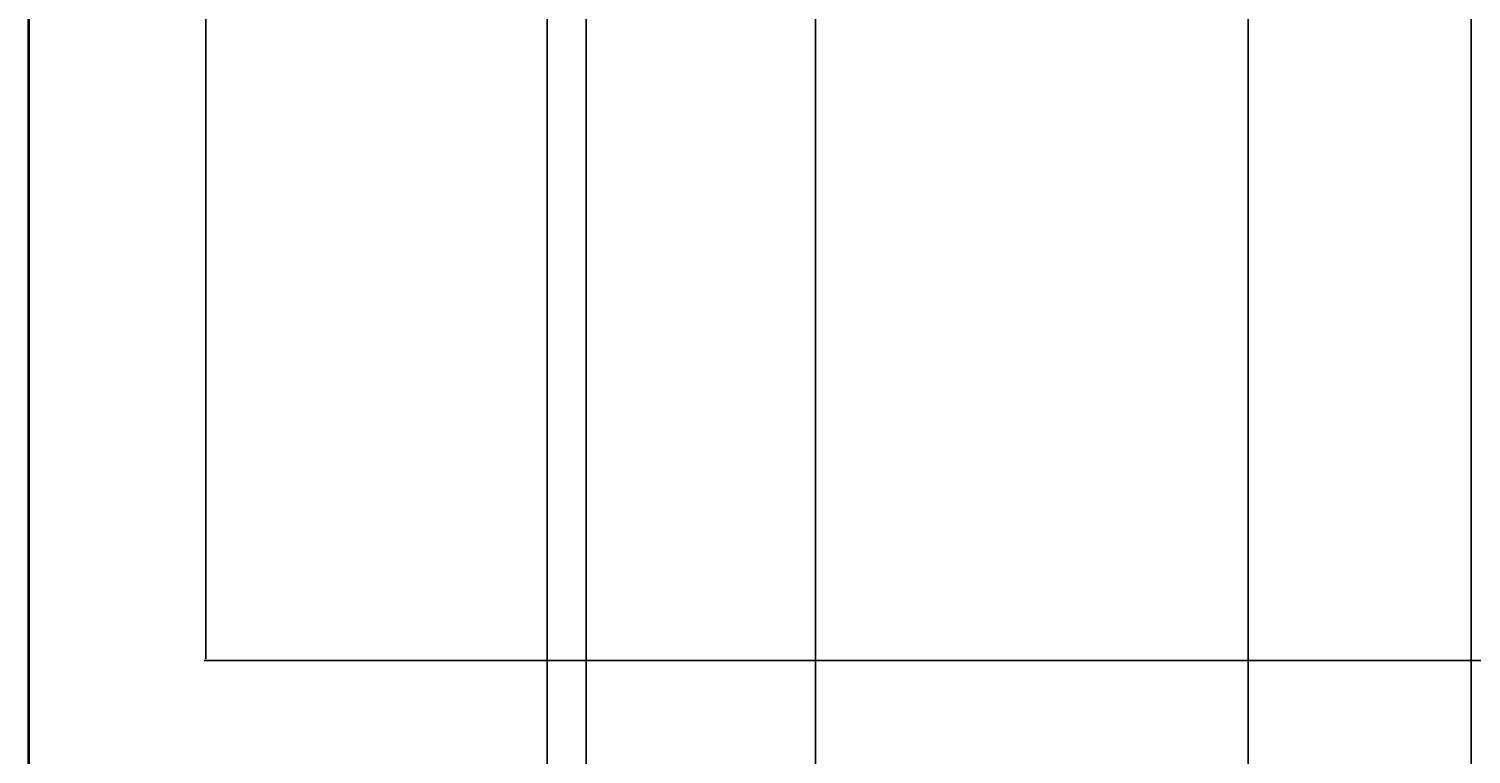
# Model space of a CAD drawing. Units: inches. Extents: x 1734 to 2405, y 1500 to 2491.
# Tile 2 of 14: x 1734 to 1900, y 1700 to 1784. Entities that reach past the tile are written whole.
import ezdxf

# ---------------------------------------------------------------- set-up
doc = ezdxf.new("R2010")
doc.units = ezdxf.units.IN
for name, color, linetype, lineweight in [('A-ANNO-DIMS', 2, 'Continuous', 18), ('A-ANNO-TTLB', 7, 'Continuous', 35), ('C-PROP', 7, 'Continuous', 25)]:
    doc.layers.add(name, color=color, linetype=linetype, lineweight=lineweight)
doc.styles.get("Standard").update_dxf_attribs({"font": 'arial.ttf'})
doc.dimstyles.get("Standard").update_dxf_attribs({"dimtxt": 0.18, "dimasz": 0.18, "dimexe": 0.18, "dimexo": 0.0625, "dimgap": 0.09, "dimtad": 0, "dimtih": 1, "dimtoh": 1, "dimdec": 4, "dimzin": 0, "dimdsep": 46, "dimtxsty": 'Standard', "dimcen": 0.09, "dimadec": 0, "dimazin": 0, "dimtfac": 1, "dimtdec": 4, "dimtofl": 0, "dimtmove": 0, "dimatfit": 3, "dimfxl": 1, "dimtolj": 1, "dimtzin": 0, "dimarcsym": 0})

# ---------------------------------------------------------------- blocks, each defined once
blk = doc.blocks.new('*D23')
at = {"layer": 'A-ANNO-DIMS', "color": 0, "lineweight": -2, "transparency": 16777216}
for p, q in [((1793.83, 2425.82), (1754.36, 2425.82)), ((1754.54, 2425.64), (1754.54, 2068.48)), ((1754.54, 1710.95), (1754.54, 2068.11)), ((1793.83, 1710.77), (1754.36, 1710.77))]:
    blk.add_line(p, q, dxfattribs=at)
at = {"layer": 'A-ANNO-DIMS', "color": 0, "transparency": 16777216}
for points in [[(1754.51, 2425.64), (1754.57, 2425.64), (1754.54, 2425.82)], [(1754.51, 1710.95), (1754.57, 1710.95), (1754.54, 1710.77)]]:
    blk.add_solid(points, dxfattribs=at)
at = {"layer": 'Defpoints', "color": 0, "transparency": 16777216}
for p in [(1754.54, 2425.82), (1793.89, 2425.82), (1793.89, 1710.77)]:
    blk.add_point(p, dxfattribs=at)
at = {"layer": 'A-ANNO-DIMS', "color": 0, "transparency": 16777216, "insert": (1754.54, 2068.3), "char_height": 0.18, "attachment_point": 5}
blk.add_mtext('\\A1;715', dxfattribs=at)
blk = doc.blocks.new('*D24')
at = {"layer": 'A-ANNO-DIMS', "color": 0, "lineweight": -2, "transparency": 16777216}
for p, q in [((1793.89, 1710.7), (1793.89, 1615.47)), ((1900.39, 1710.7), (1900.39, 1615.47)), ((1794.07, 1615.65), (1846.76, 1615.65)), ((1900.21, 1615.65), (1847.53, 1615.65))]:
    blk.add_line(p, q, dxfattribs=at)
at = {"layer": 'A-ANNO-DIMS', "color": 0, "transparency": 16777216}
for points in [[(1794.07, 1615.68), (1794.07, 1615.62), (1793.89, 1615.65)], [(1900.21, 1615.68), (1900.21, 1615.62), (1900.39, 1615.65)]]:
    blk.add_solid(points, dxfattribs=at)
at = {"layer": 'Defpoints', "color": 0, "transparency": 16777216}
for p in [(1793.89, 1710.77), (1900.39, 1710.77), (1900.39, 1615.65)]:
    blk.add_point(p, dxfattribs=at)
at = {"layer": 'A-ANNO-DIMS', "color": 0, "transparency": 16777216, "insert": (1847.14, 1615.65), "char_height": 0.18, "attachment_point": 5}
blk.add_mtext('\\A1;106.5', dxfattribs=at)
blk = doc.blocks.new('*D26')
at = {"layer": 'A-ANNO-DIMS', "color": 0, "lineweight": -2, "transparency": 16777216}
for p, q in [((1900.39, 1798.76), (1900.39, 1615.47)), ((1932.99, 1798.76), (1932.99, 1615.47)), ((1900.57, 1615.65), (1916.37, 1615.65)), ((1932.81, 1615.65), (1917.02, 1615.65))]:
    blk.add_line(p, q, dxfattribs=at)
at = {"layer": 'A-ANNO-DIMS', "color": 0, "transparency": 16777216}
for points in [[(1900.57, 1615.68), (1900.57, 1615.62), (1900.39, 1615.65)], [(1932.81, 1615.68), (1932.81, 1615.62), (1932.99, 1615.65)]]:
    blk.add_solid(points, dxfattribs=at)
at = {"layer": 'Defpoints', "color": 0, "transparency": 16777216}
for p in [(1900.39, 1798.82), (1932.99, 1798.82), (1932.99, 1615.65)]:
    blk.add_point(p, dxfattribs=at)
at = {"layer": 'A-ANNO-DIMS', "color": 0, "transparency": 16777216, "insert": (1916.69, 1615.65), "char_height": 0.18, "attachment_point": 5}
blk.add_mtext('\\A1;32.6', dxfattribs=at)
blk = doc.blocks.new('*D32')
at = {"layer": 'A-ANNO-DIMS', "color": 0, "lineweight": -2, "transparency": 16777216}
for p, q in [((1798.39, 2202.26), (1798.39, 1615.47)), ((1824.83, 2202.26), (1824.83, 1615.47)), ((1798.57, 1615.65), (1811.22, 1615.65)), ((1824.65, 1615.65), (1812.01, 1615.65))]:
    blk.add_line(p, q, dxfattribs=at)
at = {"layer": 'A-ANNO-DIMS', "color": 0, "transparency": 16777216}
for points in [[(1798.57, 1615.68), (1798.57, 1615.62), (1798.39, 1615.65)], [(1824.65, 1615.68), (1824.65, 1615.62), (1824.83, 1615.65)]]:
    blk.add_solid(points, dxfattribs=at)
at = {"layer": 'Defpoints', "color": 0, "transparency": 16777216}
for p in [(1798.39, 2202.32), (1824.83, 2202.32), (1824.83, 1615.65)]:
    blk.add_point(p, dxfattribs=at)
at = {"layer": 'A-ANNO-DIMS', "color": 0, "transparency": 16777216, "insert": (1811.61, 1615.65), "char_height": 0.18, "attachment_point": 5}
blk.add_mtext('\\A1;26.44', dxfattribs=at)
blk = doc.blocks.new('*D33')
at = {"layer": 'A-ANNO-DIMS', "color": 0, "lineweight": -2, "transparency": 16777216}
for p, q in [((1824.83, 2202.26), (1824.83, 1615.47)), ((1874.68, 2202.26), (1874.68, 1615.47)), ((1825.01, 1615.65), (1849.36, 1615.65)), ((1874.5, 1615.65), (1850.15, 1615.65))]:
    blk.add_line(p, q, dxfattribs=at)
at = {"layer": 'A-ANNO-DIMS', "color": 0, "transparency": 16777216}
for points in [[(1825.01, 1615.68), (1825.01, 1615.62), (1824.83, 1615.65)], [(1874.5, 1615.68), (1874.5, 1615.62), (1874.68, 1615.65)]]:
    blk.add_solid(points, dxfattribs=at)
at = {"layer": 'Defpoints', "color": 0, "transparency": 16777216}
for p in [(1824.83, 2202.32), (1874.68, 2202.32), (1874.68, 1615.65)]:
    blk.add_point(p, dxfattribs=at)
at = {"layer": 'A-ANNO-DIMS', "color": 0, "transparency": 16777216, "insert": (1849.76, 1615.65), "char_height": 0.18, "attachment_point": 5}
blk.add_mtext('\\A1;49.84', dxfattribs=at)

msp = doc.modelspace()

# ---------------------------------------------------------------- linework, layer by layer
at = {"layer": 'A-ANNO-TTLB'}
msp.add_lwpolyline([(1734.1307, 2491.1293), (2404.5589, 2491.1293), (2404.5589, 1500.293), (1734.1307, 1500.293)], close=True, dxfattribs=at)
at = {"layer": 'C-PROP'}
for p, q in [((1798.3942, 1900.8246), (1798.3942, 1710.7667)), ((1793.8942, 1891.8246), (1793.8942, 1710.7667)), ((1793.8942, 1710.7667), (2033.8942, 1710.7667))]:
    msp.add_line(p, q, dxfattribs=at)

# ---------------------------------------------------------------- dimensions: what is measured, and where the dimension line sits
at = {"layer": 'A-ANNO-DIMS'}
dim = msp.add_linear_dim(base=(1754.5442, 2425.8246), p1=(1793.8942, 1710.7667), p2=(1793.8942, 2425.8246), angle=90, dimstyle='Standard', override={"dimdec": 0, "dimlfac": 1, "dimrnd": 0, "dimzin": 0, "dimdsep": 46, "dimlunit": 2}, dxfattribs=at)
dim.commit()
dim.dimension.update_dxf_attribs({"geometry": '*D23', "text_midpoint": (1754.5442, 2068.2956)})
for base, p1, p2, override, picture, middle in [((1824.8343, 1615.6468), (1798.3942, 2202.3246), (1824.8343, 2202.3246), {"dimdec": 2, "dimlfac": 1, "dimrnd": 0, "dimzin": 0, "dimdsep": 46, "dimlunit": 2}, '*D32', (1811.6142, 1615.6468)), ((1874.676, 1615.6468), (1824.8343, 2202.3246), (1874.676, 2202.3246), {"dimdec": 2, "dimlfac": 1, "dimrnd": 0, "dimzin": 0, "dimdsep": 46, "dimlunit": 2}, '*D33', (1849.7551, 1615.6468)), ((1932.9923, 1615.6468), (1900.3942, 1798.8246), (1932.9923, 1798.8246), {"dimdec": 1, "dimlfac": 1, "dimrnd": 0, "dimzin": 0, "dimdsep": 46, "dimlunit": 2}, '*D26', (1916.6932, 1615.6468)), ((1900.3942, 1615.6468), (1793.8942, 1710.7667), (1900.3942, 1710.7667), {"dimdec": 1, "dimlfac": 1, "dimrnd": 0, "dimzin": 0, "dimdsep": 46, "dimlunit": 2}, '*D24', (1847.1442, 1615.6468))]:
    dim = msp.add_linear_dim(base=base, p1=p1, p2=p2, dimstyle='Standard', override=override, dxfattribs=at)
    dim.commit()
    dim.dimension.update_dxf_attribs({"geometry": picture, "text_midpoint": middle})

doc.saveas('drawing.dxf')
